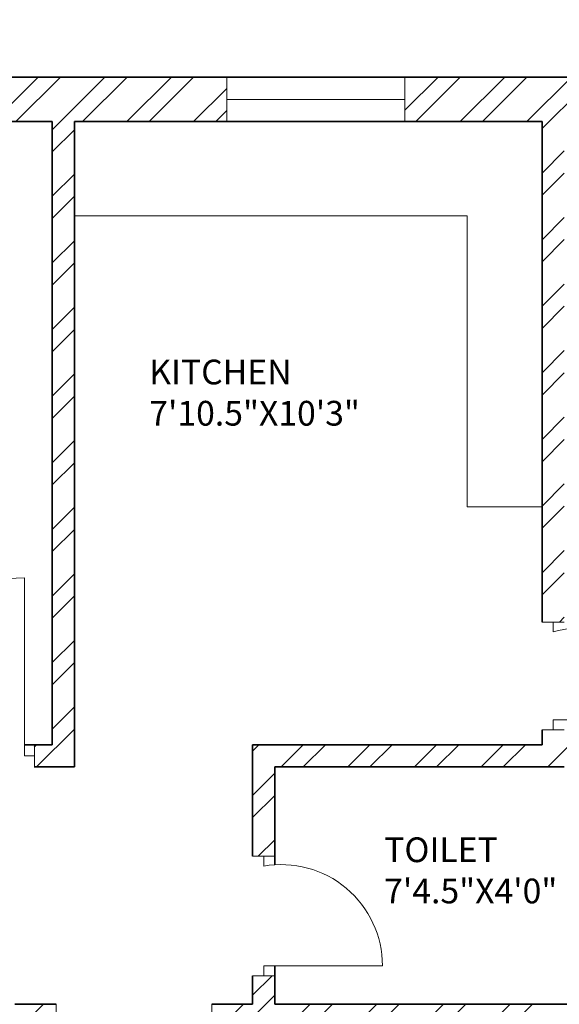
# Model space of a CAD drawing. Units: inches. Extents: x 2120 to 4013, y 1390 to 3019.
# Tile 44 of 59: x 2861 to 2970, y 2165 to 2364. Entities that reach past the tile are written whole.
import ezdxf

# ---------------------------------------------------------------- set-up
doc = ezdxf.new("R2010")
doc.units = ezdxf.units.IN
for name, color, linetype, lineweight in [('A-ANNO-DIMS', 2, 'Continuous', 18), ('A-AREA-IDEN', 7, 'Continuous', 18), ('A-DOOR', 3, 'Continuous', 18), ('A-FLOR-CASE', 8, 'Continuous', 18), ('A-GLAZ', 4, 'Continuous', 18), ('A-WALL', 7, 'Continuous', 35), ('A-WALL-PATT', 252, 'Continuous', 13)]:
    doc.layers.add(name, color=color, linetype=linetype, lineweight=lineweight)
doc.styles.get("Standard").update_dxf_attribs({"font": 'arial.ttf'})
doc.dimstyles.get("Standard").update_dxf_attribs({"dimtxt": 0.18, "dimasz": 0.18, "dimexe": 0.18, "dimexo": 0.0625, "dimgap": 0.09, "dimtad": 0, "dimtih": 1, "dimtoh": 1, "dimdec": 4, "dimzin": 0, "dimdsep": 46, "dimtxsty": 'Standard', "dimcen": 0.09, "dimadec": 0, "dimazin": 0, "dimtfac": 1, "dimtdec": 4, "dimtofl": 0, "dimtmove": 0, "dimatfit": 3, "dimfxl": 1, "dimtolj": 1, "dimtzin": 0, "dimarcsym": 0})

# ---------------------------------------------------------------- blocks, each defined once
blk = doc.blocks.new('DOOR-SWING-24IN-106p92DEG')
for p, q in [((4.5, 21.79), (0, 21.79)), ((0, 21.79), (2.25, 21.79)), ((2.25, 21.79), (2.25, 19.79)), ((2.25, 0), (2.25, 2)), ((2.25, 2), (26.25, 2)), ((0, 0), (4.5, 0)), ((4.5, 0), (2.25, 0))]:
    blk.add_line(p, q)
blk.add_arc((7.66, 2), 18.59, 0, 106.9181)
blk = doc.blocks.new('DOOR-SWING-24IN-99p98DEG')
for p, q in [((0, 24.15), (4.5, 24.15)), ((4.5, 24.15), (2.25, 24.15)), ((2.25, 24.15), (2.25, 22.15)), ((2.25, 0), (2.25, 2)), ((2.25, 2), (26.25, 2)), ((4.5, 0), (0, 0)), ((0, 0), (2.25, 0))]:
    blk.add_line(p, q)
blk.add_arc((5.79, 2), 20.46, 0, 99.9792)
blk = doc.blocks.new('DOOR-SWING-36IN-103p63DEG')
for p, q in [((30.32, 2.25), (30.32, 38.25)), ((0, 4.5), (0, 0)), ((32.32, 4.5), (32.32, 0)), ((0, 0), (0, 2.25)), ((0, 2.25), (2, 2.25)), ((32.32, 2.25), (30.32, 2.25)), ((32.32, 0), (32.32, 2.25))]:
    blk.add_line(p, q)
blk.add_arc((30.32, 9.11), 29.14, 90, 193.6269)
blk = doc.blocks.new('DOOR-SWING-36IN-105p32DEG')
for p, q in [((0, 33.75), (0, 38.25)), ((0, 38.25), (0, 36)), ((31.46, 33.75), (31.46, 38.25)), ((31.46, 38.25), (31.46, 36)), ((0, 36), (2, 36)), ((2, 36), (2, 0)), ((31.46, 36), (29.46, 36))]:
    blk.add_line(p, q)
blk.add_arc((2, 28.48), 28.48, 270, 15.3194)
blk = doc.blocks.new('WIN-PLAN-36IN')
for p, q in [((0, 0), (0, 9)), ((0, 9), (0, 4.5)), ((36, 4.5), (36, 9)), ((36, 9), (36, 0)), ((0, 4.5), (36, 4.5))]:
    blk.add_line(p, q)
blk = doc.blocks.new('*D211')
at = {"layer": 'A-ANNO-DIMS', "color": 0, "lineweight": -2, "transparency": 16777216}
for p, q in [((2262.73, 2352.59), (2262.73, 2397.71)), ((2262.91, 2397.53), (2635.95, 2397.53)), ((3009.55, 2397.53), (2636.52, 2397.53)), ((3009.73, 2352.59), (3009.73, 2397.71))]:
    blk.add_line(p, q, dxfattribs=at)
at = {"layer": 'A-ANNO-DIMS', "color": 0, "transparency": 16777216}
for points in [[(2262.91, 2397.56), (2262.91, 2397.5), (2262.73, 2397.53)], [(3009.55, 2397.56), (3009.55, 2397.5), (3009.73, 2397.53)]]:
    blk.add_solid(points, dxfattribs=at)
at = {"layer": 'Defpoints', "color": 0, "transparency": 16777216}
for p in [(3009.73, 2397.53), (2262.73, 2352.53), (3009.73, 2352.53)]:
    blk.add_point(p, dxfattribs=at)
at = {"layer": 'A-ANNO-DIMS', "color": 0, "transparency": 16777216, "insert": (2636.23, 2397.53), "char_height": 0.18, "attachment_point": 5}
blk.add_mtext('\\A1;747', dxfattribs=at)

msp = doc.modelspace()

# ---------------------------------------------------------------- hatches: boundary and pattern name
at = {"layer": 'A-WALL-PATT'}
h = msp.add_hatch(dxfattribs=at)
h.set_pattern_fill('ANSI32', color=256)
h.paths.add_polyline_path([(2271.7331, 2343.531), (2283.3788, 2343.531), (2283.3788, 2348.031), (2283.3788, 2352.5306), (2262.7331, 2352.5306), (2262.7331, 2182.638), (2267.2331, 2182.638), (2271.7331, 2182.638), (2271.7331, 2219.031), (2391.7331, 2219.031), (2391.7331, 2214.189), (2393.9831, 2214.189), (2396.2331, 2214.189), (2396.2331, 2219.031), (2420.2331, 2219.031), (2420.2331, 2225.7535), (2417.2197, 2225.7535), (2415.7331, 2225.7535), (2415.7331, 2223.5306), (2271.7331, 2223.5306)])
h.paths.add_polyline_path([(2380.0942, 2352.5306), (2343.3788, 2352.5306), (2343.3788, 2343.531), (2363.2331, 2343.531), (2363.2331, 2288.8489), (2365.4831, 2288.8489), (2367.7331, 2288.8489), (2367.7331, 2343.531), (2380.0942, 2343.531)], flags=17)
h.paths.add_polyline_path([(2432.4339, 2352.5306), (2404.0943, 2352.5306), (2404.0943, 2343.531), (2415.7331, 2343.531), (2415.7331, 2264.0306), (2367.7331, 2264.0306), (2367.7331, 2266.4872), (2363.2331, 2266.4872), (2363.2331, 2259.531), (2367.7331, 2259.531), (2415.7331, 2259.531), (2415.7331, 2255.0658), (2420.2331, 2255.0658), (2420.2331, 2259.531), (2424.5717, 2259.531), (2424.5717, 2261.781), (2424.5717, 2264.0306), (2420.2331, 2264.0306), (2420.2331, 2343.531), (2432.4339, 2343.531)])
h.paths.add_polyline_path([(2508.9115, 2352.5306), (2456.4339, 2352.5306), (2456.4339, 2343.531), (2468.2331, 2343.531), (2468.2331, 2264.0306), (2448.0487, 2264.0306), (2448.0487, 2259.531), (2468.2331, 2259.531), (2468.2331, 2255.5496), (2472.7331, 2255.5496), (2472.7331, 2343.531), (2508.9115, 2343.531)])
h.paths.add_polyline_path([(2637.7331, 2352.5306), (2544.9116, 2352.5306), (2544.9116, 2343.531), (2589.7331, 2343.531), (2633.2331, 2343.531), (2637.7331, 2343.531)])
h.paths.add_polyline_path([(2594.2331, 2343.5306), (2589.7331, 2343.5306), (2589.7331, 2259.5306), (2589.7331, 2252.4915), (2591.9831, 2252.4915), (2594.2331, 2252.4915)])
h.paths.add_polyline_path([(2637.7331, 2223.5306), (2594.2331, 2223.5306), (2594.2331, 2230.1988), (2591.9831, 2230.1988), (2589.7331, 2230.1988), (2589.7331, 2223.5306), (2472.7331, 2223.5306), (2468.2331, 2223.5306), (2468.2331, 2219.031), (2628.7331, 2219.031), (2628.7331, 2138.031), (2637.7331, 2138.031)])
h.paths.add_polyline_path([(3822.6535, 2458.4402), (3874.9468, 2458.4402), (3874.9468, 2476.9866), (3822.6535, 2476.9866)], flags=9)
h.paths.add_polyline_path([(3834.6921, 2781.8174), (3935.9206, 2781.8174), (3935.9206, 2800.3638), (3834.6921, 2800.3638)], flags=9)
h.paths.add_polyline_path([(3832.2843, 2837.9683), (3884.5776, 2837.9683), (3884.5776, 2856.5146), (3832.2843, 2856.5146)], flags=9)
h.paths.add_polyline_path([(3830.9388, 2861.4782), (3956.8958, 2861.4782), (3956.8958, 2880.0245), (3830.9388, 2880.0245)], flags=9)
h.paths.add_polyline_path([(3870.6966, 2352.5752), (3887.9272, 2352.5752), (3887.9272, 2377.3037), (3870.6966, 2377.3037)], flags=9)
h.paths.add_polyline_path([(3289.2701, 2413.161), (3435.2223, 2413.161), (3435.2223, 2450.2538), (3289.2701, 2450.2538)], flags=9)
h.paths.add_polyline_path([(2487.6944, 2414.3601), (2637.8335, 2414.3601), (2637.8335, 2451.4528), (2487.6944, 2451.4528)], flags=9)
h.paths.add_polyline_path([(2567.3724, 1457.9199), (2815.296, 1457.9199), (2815.296, 1495.0127), (2567.3724, 1495.0127)], flags=9)
h.paths.add_polyline_path([(2655.3825, 2093.2363), (2685.9555, 2093.2363), (2685.9555, 2111.8937), (2655.3825, 2111.8937)], flags=9)
h.paths.add_polyline_path([(2543.9218, 1550.6671), (2587.8406, 1550.6671), (2587.8406, 1569.3244), (2543.9218, 1569.3244)], flags=9)
h.paths.add_polyline_path([(2905.1384, 1543.8113), (2949.0572, 1543.8113), (2949.0572, 1562.4686), (2905.1384, 1562.4686)], flags=9)
h.paths.add_polyline_path([(2736.4118, 1702.4736), (2784.2153, 1702.4736), (2784.2153, 1721.1309), (2736.4118, 1721.1309)], flags=9)
h.paths.add_polyline_path([(2912.8666, 1710.4168), (2951.707, 1710.4168), (2951.707, 1729.0741), (2912.8666, 1729.0741)], flags=9)
h.paths.add_polyline_path([(2923.5785, 1763.5038), (2959.7279, 1763.5038), (2959.7279, 1782.1611), (2923.5785, 1782.1611)], flags=9)
h.paths.add_polyline_path([(2925.2114, 1809.6137), (2967.1861, 1809.6137), (2967.1861, 1828.271), (2925.2114, 1828.271)], flags=9)
h.paths.add_polyline_path([(2996.2711, 1878.9003), (2996.2711, 1913.109), (2977.6138, 1913.109), (2977.6138, 1878.9003)], flags=9)
h.paths.add_polyline_path([(2883.0859, 1895.7192), (2927.1855, 1895.7192), (2927.1855, 1914.3766), (2883.0859, 1914.3766)], flags=9)
h.paths.add_polyline_path([(2787.3924, 1810.8013), (2841.0213, 1810.8013), (2841.0213, 1829.4587), (2787.3924, 1829.4587)], flags=9)
h.paths.add_polyline_path([(2775.6399, 2101.7395), (2829.2689, 2101.7395), (2829.2689, 2120.3968), (2775.6399, 2120.3968)], flags=9)
h.paths.add_polyline_path([(2913.0263, 2075.817), (2951.8667, 2075.817), (2951.8667, 2094.4744), (2913.0263, 2094.4744)], flags=9)
h.paths.add_polyline_path([(2929.966, 2133.3669), (2966.1154, 2133.3669), (2966.1154, 2152.0243), (2929.966, 2152.0243)], flags=9)
h.paths.add_polyline_path([(2932.7502, 2182.6088), (2968.8996, 2182.6088), (2968.8996, 2201.2662), (2932.7502, 2201.2662)], flags=9)
h.paths.add_polyline_path([(2996.0681, 2266.3173), (2996.0681, 2300.5261), (2977.4108, 2300.5261), (2977.4108, 2266.3173)], flags=9)
h.paths.add_polyline_path([(2885.1039, 2279.2186), (2929.2035, 2279.2186), (2929.2035, 2297.8759), (2885.1039, 2297.8759)], flags=9)
h.paths.add_polyline_path([(2735.7042, 2218.3197), (2783.5078, 2218.3197), (2783.5078, 2236.9771), (2735.7042, 2236.9771)], flags=9)
h.paths.add_polyline_path([(2635.6049, 2044.0085), (2648.9678, 2044.0085), (2648.9678, 2054.312), (2635.6049, 2054.312)], flags=9)
h.paths.add_polyline_path([(2714.0148, 1923.0473), (2727.3777, 1923.0473), (2727.3777, 1933.3508), (2714.0148, 1933.3508)], flags=9)
h.paths.add_polyline_path([(2709.0345, 1988.1628), (2722.3974, 1988.1628), (2722.3974, 1998.4663), (2709.0345, 1998.4663)], flags=9)
h.paths.add_polyline_path([(2592.8935, 1962.1763), (2606.2564, 1962.1763), (2606.2564, 1972.4799), (2592.8935, 1972.4799)], flags=9)
h.paths.add_polyline_path([(2618.3996, 1985.9724), (2644.1942, 1985.9724), (2644.1942, 1996.2759), (2618.3996, 1996.2759)], flags=9)
h.paths.add_polyline_path([(2601.279, 1920.5869), (2614.6419, 1920.5869), (2614.6419, 1930.8904), (2601.279, 1930.8904)], flags=9)
h.paths.add_polyline_path([(2692.3278, 1932.7645), (2704.5311, 1932.7645), (2704.5311, 1943.0681), (2692.3278, 1943.0681)], flags=9)
h.paths.add_polyline_path([(2311.122, 1672.7318), (2355.0408, 1672.7318), (2355.0408, 1691.3892), (2311.122, 1691.3892)], flags=9)
h.paths.add_polyline_path([(2456.2551, 1632.3198), (2492.4796, 1632.3198), (2492.4796, 1650.9772), (2456.2551, 1650.9772)], flags=9)
h.paths.add_polyline_path([(2401.0766, 1631.4793), (2437.301, 1631.4793), (2437.301, 1650.1367), (2401.0766, 1650.1367)], flags=9)
h.paths.add_polyline_path([(2546.7054, 1700.9235), (2594.509, 1700.9235), (2594.509, 1719.5809), (2546.7054, 1719.5809)], flags=9)
h.paths.add_polyline_path([(2445.4866, 1766.9937), (2497.5261, 1766.9937), (2497.5261, 1785.651), (2445.4866, 1785.651)], flags=9)
h.paths.add_polyline_path([(2287.9992, 1739.7675), (2326.8396, 1739.7675), (2326.8396, 1758.4248), (2287.9992, 1758.4248)], flags=9)
h.paths.add_polyline_path([(2458.5279, 1924.7607), (2510.5675, 1924.7607), (2510.5675, 1943.4181), (2458.5279, 1943.4181)], flags=9)
h.paths.add_polyline_path([(2309.2811, 1902.7642), (2345.4305, 1902.7642), (2345.4305, 1921.4215), (2309.2811, 1921.4215)], flags=9)
h.paths.add_polyline_path([(2490.7554, 2018.9392), (2530.7896, 2018.9392), (2530.7896, 2037.5965), (2490.7554, 2037.5965)], flags=9)
h.paths.add_polyline_path([(2402.143, 2024.7393), (2438.5414, 2024.7393), (2438.5414, 2043.3966), (2402.143, 2043.3966)], flags=9)
h.paths.add_polyline_path([(2287.856, 1931.7926), (2326.6964, 1931.7926), (2326.6964, 1950.4499), (2287.856, 1950.4499)], flags=9)
h.paths.add_polyline_path([(2281.7979, 2193.5771), (2320.6383, 2193.5771), (2320.6383, 2212.2344), (2281.7979, 2212.2344)], flags=25)
h.paths.add_polyline_path([(2484.0754, 2093.892), (2536.115, 2093.892), (2536.115, 2112.5494), (2484.0754, 2112.5494)], flags=9)
h.paths.add_polyline_path([(2624.7948, 2281.8639), (2624.7948, 2311.4137), (2606.1375, 2311.4137), (2606.1375, 2281.8639)], flags=9)
h.paths.add_polyline_path([(2507.5036, 2290.3639), (2541.934, 2290.3639), (2541.934, 2309.0212), (2507.5036, 2309.0212)], flags=9)
h.paths.add_polyline_path([(2423.1076, 2285.2202), (2459.332, 2285.2202), (2459.332, 2303.8776), (2423.1076, 2303.8776)], flags=9)
h.paths.add_polyline_path([(2374.5467, 2289.6272), (2410.7711, 2289.6272), (2410.7711, 2308.2846), (2374.5467, 2308.2846)], flags=25)
h.paths.add_polyline_path([(2277.4907, 2227.5651), (2316.3311, 2227.5651), (2316.3311, 2246.2224), (2277.4907, 2246.2224)], flags=25)
h.paths.add_polyline_path([(2655.3825, 2093.2367), (2685.9555, 2093.2367), (2685.9555, 2111.894), (2655.3825, 2111.894)], flags=9)
h.paths.add_polyline_path([(2543.9217, 1550.6674), (2587.8406, 1550.6674), (2587.8406, 1569.3247), (2543.9217, 1569.3247)], flags=9)
h.paths.add_polyline_path([(2905.1384, 1543.8116), (2949.0572, 1543.8116), (2949.0572, 1562.4689), (2905.1384, 1562.4689)], flags=9)
h.paths.add_polyline_path([(2736.4118, 1702.4739), (2784.2153, 1702.4739), (2784.2153, 1721.1312), (2736.4118, 1721.1312)], flags=9)
h.paths.add_polyline_path([(2912.8666, 1710.4171), (2951.707, 1710.4171), (2951.707, 1729.0744), (2912.8666, 1729.0744)], flags=9)
h.paths.add_polyline_path([(2923.5785, 1763.5041), (2959.7279, 1763.5041), (2959.7279, 1782.1614), (2923.5785, 1782.1614)], flags=9)
h.paths.add_polyline_path([(2925.2114, 1809.614), (2967.1861, 1809.614), (2967.1861, 1828.2713), (2925.2114, 1828.2713)], flags=9)
h.paths.add_polyline_path([(2996.2711, 1878.9006), (2996.2711, 1913.1094), (2977.6137, 1913.1094), (2977.6137, 1878.9006)], flags=9)
h.paths.add_polyline_path([(2883.0859, 1895.7195), (2927.1855, 1895.7195), (2927.1855, 1914.3769), (2883.0859, 1914.3769)], flags=9)
h.paths.add_polyline_path([(2787.3924, 1810.8016), (2841.0213, 1810.8016), (2841.0213, 1829.459), (2787.3924, 1829.459)], flags=9)
h.paths.add_polyline_path([(2775.6399, 2101.7398), (2829.2688, 2101.7398), (2829.2688, 2120.3971), (2775.6399, 2120.3971)], flags=9)
h.paths.add_polyline_path([(2913.0263, 2075.8173), (2951.8667, 2075.8173), (2951.8667, 2094.4747), (2913.0263, 2094.4747)], flags=9)
h.paths.add_polyline_path([(2929.966, 2133.3672), (2966.1154, 2133.3672), (2966.1154, 2152.0246), (2929.966, 2152.0246)], flags=9)
h.paths.add_polyline_path([(2932.7502, 2182.6091), (2968.8996, 2182.6091), (2968.8996, 2201.2665), (2932.7502, 2201.2665)], flags=9)
h.paths.add_polyline_path([(2996.0681, 2266.3176), (2996.0681, 2300.5264), (2977.4108, 2300.5264), (2977.4108, 2266.3176)], flags=9)
h.paths.add_polyline_path([(2885.1039, 2279.2189), (2929.2035, 2279.2189), (2929.2035, 2297.8762), (2885.1039, 2297.8762)], flags=9)
h.paths.add_polyline_path([(2735.7042, 2218.32), (2783.5078, 2218.32), (2783.5078, 2236.9774), (2735.7042, 2236.9774)], flags=9)
h.paths.add_polyline_path([(2635.6048, 2044.0088), (2648.9677, 2044.0088), (2648.9677, 2054.3123), (2635.6048, 2054.3123)], flags=9)
h.paths.add_polyline_path([(2714.0148, 1923.0476), (2727.3777, 1923.0476), (2727.3777, 1933.3511), (2714.0148, 1933.3511)], flags=9)
h.paths.add_polyline_path([(2709.0345, 1988.1631), (2722.3974, 1988.1631), (2722.3974, 1998.4666), (2709.0345, 1998.4666)], flags=9)
h.paths.add_polyline_path([(2592.8935, 1962.1766), (2606.2564, 1962.1766), (2606.2564, 1972.4802), (2592.8935, 1972.4802)], flags=9)
h.paths.add_polyline_path([(2618.3995, 1985.9727), (2644.1942, 1985.9727), (2644.1942, 1996.2762), (2618.3995, 1996.2762)], flags=9)
h.paths.add_polyline_path([(2601.279, 1920.5872), (2614.6419, 1920.5872), (2614.6419, 1930.8908), (2601.279, 1930.8908)], flags=9)
h.paths.add_polyline_path([(2692.3278, 1932.7648), (2704.5311, 1932.7648), (2704.5311, 1943.0684), (2692.3278, 1943.0684)], flags=9)
h.paths.add_polyline_path([(2311.122, 1672.7321), (2355.0408, 1672.7321), (2355.0408, 1691.3895), (2311.122, 1691.3895)], flags=9)
h.paths.add_polyline_path([(2456.2551, 1632.3201), (2492.4795, 1632.3201), (2492.4795, 1650.9775), (2456.2551, 1650.9775)], flags=9)
h.paths.add_polyline_path([(2401.0766, 1631.4796), (2437.301, 1631.4796), (2437.301, 1650.137), (2401.0766, 1650.137)], flags=9)
h.paths.add_polyline_path([(2546.7054, 1700.9238), (2594.509, 1700.9238), (2594.509, 1719.5812), (2546.7054, 1719.5812)], flags=9)
h.paths.add_polyline_path([(2445.4866, 1766.994), (2497.5261, 1766.994), (2497.5261, 1785.6513), (2445.4866, 1785.6513)], flags=9)
h.paths.add_polyline_path([(2287.9992, 1739.7678), (2326.8396, 1739.7678), (2326.8396, 1758.4251), (2287.9992, 1758.4251)], flags=9)
h.paths.add_polyline_path([(2458.5279, 1924.7611), (2510.5675, 1924.7611), (2510.5675, 1943.4184), (2458.5279, 1943.4184)], flags=9)
h.paths.add_polyline_path([(2309.2811, 1902.7645), (2345.4305, 1902.7645), (2345.4305, 1921.4218), (2309.2811, 1921.4218)], flags=9)
h.paths.add_polyline_path([(2490.7554, 2018.9395), (2530.7895, 2018.9395), (2530.7895, 2037.5968), (2490.7554, 2037.5968)], flags=9)
h.paths.add_polyline_path([(2402.143, 2024.7396), (2438.5413, 2024.7396), (2438.5413, 2043.3969), (2402.143, 2043.3969)], flags=9)
h.paths.add_polyline_path([(2287.856, 1931.7929), (2326.6964, 1931.7929), (2326.6964, 1950.4502), (2287.856, 1950.4502)], flags=9)
h.paths.add_polyline_path([(2281.7979, 2193.5774), (2320.6383, 2193.5774), (2320.6383, 2212.2347), (2281.7979, 2212.2347)], flags=25)
h.paths.add_polyline_path([(2484.0754, 2093.8924), (2536.115, 2093.8924), (2536.115, 2112.5497), (2484.0754, 2112.5497)], flags=9)
h.paths.add_polyline_path([(2624.7948, 2281.8642), (2624.7948, 2311.414), (2606.1374, 2311.414), (2606.1374, 2281.8642)], flags=9)
h.paths.add_polyline_path([(2507.5035, 2290.3642), (2541.934, 2290.3642), (2541.934, 2309.0215), (2507.5035, 2309.0215)], flags=9)
h.paths.add_polyline_path([(2423.1075, 2285.2205), (2459.332, 2285.2205), (2459.332, 2303.8779), (2423.1075, 2303.8779)], flags=9)
h.paths.add_polyline_path([(2374.5467, 2289.6275), (2410.7711, 2289.6275), (2410.7711, 2308.2849), (2374.5467, 2308.2849)], flags=25)
h.paths.add_polyline_path([(2277.4907, 2227.5654), (2316.3311, 2227.5654), (2316.3311, 2246.2227), (2277.4907, 2246.2227)], flags=25)
h = msp.add_hatch(dxfattribs=at)
h.set_pattern_fill('ANSI32', color=256)
h.paths.add_polyline_path([(2271.7331, 1980.389), (2262.7331, 1980.389), (2262.7331, 1912.8434), (2267.2331, 1912.8434), (2271.7331, 1912.8434), (2271.7331, 1922.531), (2351.2331, 1922.531), (2351.2331, 1901.4728), (2355.7331, 1901.4728), (2355.7331, 1922.531), (2357.9815, 1922.531), (2357.9815, 1926.5306), (2271.7331, 1926.5306)])
h.paths.add_polyline_path([(2589.2331, 1949.1622), (2584.7331, 1949.1622), (2580.2331, 1949.1622), (2580.2331, 1874.5306), (2355.7331, 1874.5306), (2355.7331, 1880.1922), (2351.2331, 1880.1922), (2351.2331, 1874.5306), (2271.7331, 1874.5306), (2271.7331, 1888.8431), (2262.7331, 1888.8431), (2262.7331, 1842.2909), (2267.2331, 1842.2909), (2271.7331, 1842.2909), (2271.7331, 1865.531), (2415.7331, 1865.531), (2415.7331, 1779.7286), (2420.2331, 1779.7286), (2420.2331, 1865.531), (2589.2331, 1865.531)])
h.paths.add_polyline_path([(2271.7331, 1782.2906), (2262.7331, 1782.2906), (2262.7331, 1711.4639), (2267.2331, 1711.4639), (2271.7331, 1711.4639), (2271.7331, 1738.031), (2420.2331, 1738.031), (2420.2331, 1742.531), (2420.2331, 1747.3376), (2417.9831, 1747.3376), (2415.7331, 1747.3376), (2415.7331, 1742.5306), (2271.7331, 1742.5306)])
h.paths.add_polyline_path([(2271.7331, 1627.031), (2362.3957, 1627.031), (2362.3957, 1629.281), (2362.3957, 1631.5306), (2271.7331, 1631.5306), (2271.7331, 1675.4636), (2262.7331, 1675.4636), (2262.7331, 1581.531), (2405.3032, 1581.531), (2405.3032, 1586.031), (2405.3032, 1590.5306), (2396.2331, 1590.5306), (2396.2331, 1691.4513), (2418.7206, 1691.4513), (2418.7206, 1695.951), (2396.2331, 1695.951), (2391.7331, 1695.951), (2391.7331, 1631.5306), (2386.7425, 1631.5306), (2386.7425, 1629.2806), (2386.7425, 1627.031), (2391.7331, 1627.031), (2391.7331, 1586.1709), (2271.7331, 1586.1709)])
h.paths.add_polyline_path([(2459.6703, 1590.5306), (2429.3032, 1590.5306), (2429.3032, 1581.531), (2459.6703, 1581.531), (2459.6703, 1586.031)])
h.paths.add_polyline_path([(2501.2331, 1590.531), (2501.2331, 1665.0195), (2498.9831, 1665.0195), (2496.7331, 1665.0195), (2496.7331, 1590.5306), (2483.8201, 1590.5306), (2483.8201, 1590.1579), (2483.6704, 1590.1579), (2483.6704, 1581.531), (2505.0196, 1581.531), (2505.0196, 1583.781), (2505.0196, 1586.0306), (2501.2331, 1586.0306)])
h.paths.add_polyline_path([(2544.1361, 1583.781), (2544.1361, 1586.0306), (2527.1368, 1586.0306), (2527.1368, 1583.7806), (2527.1368, 1581.531), (2544.1361, 1581.531)])
h.paths.add_polyline_path([(3822.6535, 2458.4402), (3874.9468, 2458.4402), (3874.9468, 2476.9866), (3822.6535, 2476.9866)], flags=9)
h.paths.add_polyline_path([(3834.6921, 2781.8174), (3935.9206, 2781.8174), (3935.9206, 2800.3638), (3834.6921, 2800.3638)], flags=9)
h.paths.add_polyline_path([(3832.2843, 2837.9683), (3884.5776, 2837.9683), (3884.5776, 2856.5146), (3832.2843, 2856.5146)], flags=9)
h.paths.add_polyline_path([(3830.9388, 2861.4782), (3956.8958, 2861.4782), (3956.8958, 2880.0245), (3830.9388, 2880.0245)], flags=9)
h.paths.add_polyline_path([(3870.6966, 2352.5752), (3887.9272, 2352.5752), (3887.9272, 2377.3037), (3870.6966, 2377.3037)], flags=9)
h.paths.add_polyline_path([(3289.2701, 2413.161), (3435.2223, 2413.161), (3435.2223, 2450.2538), (3289.2701, 2450.2538)], flags=9)
h.paths.add_polyline_path([(2487.6944, 2414.3601), (2637.8335, 2414.3601), (2637.8335, 2451.4528), (2487.6944, 2451.4528)], flags=9)
h.paths.add_polyline_path([(2567.3724, 1457.9199), (2815.296, 1457.9199), (2815.296, 1495.0127), (2567.3724, 1495.0127)], flags=9)
h.paths.add_polyline_path([(2655.3825, 2093.2363), (2685.9555, 2093.2363), (2685.9555, 2111.8937), (2655.3825, 2111.8937)], flags=9)
h.paths.add_polyline_path([(2543.9218, 1550.6671), (2587.8406, 1550.6671), (2587.8406, 1569.3244), (2543.9218, 1569.3244)], flags=9)
h.paths.add_polyline_path([(2905.1384, 1543.8113), (2949.0572, 1543.8113), (2949.0572, 1562.4686), (2905.1384, 1562.4686)], flags=9)
h.paths.add_polyline_path([(2736.4118, 1702.4736), (2784.2153, 1702.4736), (2784.2153, 1721.1309), (2736.4118, 1721.1309)], flags=9)
h.paths.add_polyline_path([(2912.8666, 1710.4168), (2951.707, 1710.4168), (2951.707, 1729.0741), (2912.8666, 1729.0741)], flags=9)
h.paths.add_polyline_path([(2923.5785, 1763.5038), (2959.7279, 1763.5038), (2959.7279, 1782.1611), (2923.5785, 1782.1611)], flags=9)
h.paths.add_polyline_path([(2925.2114, 1809.6137), (2967.1861, 1809.6137), (2967.1861, 1828.271), (2925.2114, 1828.271)], flags=9)
h.paths.add_polyline_path([(2996.2711, 1878.9003), (2996.2711, 1913.109), (2977.6138, 1913.109), (2977.6138, 1878.9003)], flags=9)
h.paths.add_polyline_path([(2883.0859, 1895.7192), (2927.1855, 1895.7192), (2927.1855, 1914.3766), (2883.0859, 1914.3766)], flags=9)
h.paths.add_polyline_path([(2787.3924, 1810.8013), (2841.0213, 1810.8013), (2841.0213, 1829.4587), (2787.3924, 1829.4587)], flags=9)
h.paths.add_polyline_path([(2775.6399, 2101.7395), (2829.2689, 2101.7395), (2829.2689, 2120.3968), (2775.6399, 2120.3968)], flags=9)
h.paths.add_polyline_path([(2913.0263, 2075.817), (2951.8667, 2075.817), (2951.8667, 2094.4744), (2913.0263, 2094.4744)], flags=9)
h.paths.add_polyline_path([(2929.966, 2133.3669), (2966.1154, 2133.3669), (2966.1154, 2152.0243), (2929.966, 2152.0243)], flags=9)
h.paths.add_polyline_path([(2932.7502, 2182.6088), (2968.8996, 2182.6088), (2968.8996, 2201.2662), (2932.7502, 2201.2662)], flags=9)
h.paths.add_polyline_path([(2996.0681, 2266.3173), (2996.0681, 2300.5261), (2977.4108, 2300.5261), (2977.4108, 2266.3173)], flags=9)
h.paths.add_polyline_path([(2885.1039, 2279.2186), (2929.2035, 2279.2186), (2929.2035, 2297.8759), (2885.1039, 2297.8759)], flags=9)
h.paths.add_polyline_path([(2735.7042, 2218.3197), (2783.5078, 2218.3197), (2783.5078, 2236.9771), (2735.7042, 2236.9771)], flags=9)
h.paths.add_polyline_path([(2635.6049, 2044.0085), (2648.9678, 2044.0085), (2648.9678, 2054.312), (2635.6049, 2054.312)], flags=9)
h.paths.add_polyline_path([(2714.0148, 1923.0473), (2727.3777, 1923.0473), (2727.3777, 1933.3508), (2714.0148, 1933.3508)], flags=9)
h.paths.add_polyline_path([(2709.0345, 1988.1628), (2722.3974, 1988.1628), (2722.3974, 1998.4663), (2709.0345, 1998.4663)], flags=9)
h.paths.add_polyline_path([(2592.8935, 1962.1763), (2606.2564, 1962.1763), (2606.2564, 1972.4799), (2592.8935, 1972.4799)], flags=9)
h.paths.add_polyline_path([(2618.3996, 1985.9724), (2644.1942, 1985.9724), (2644.1942, 1996.2759), (2618.3996, 1996.2759)], flags=9)
h.paths.add_polyline_path([(2601.279, 1920.5869), (2614.6419, 1920.5869), (2614.6419, 1930.8904), (2601.279, 1930.8904)], flags=9)
h.paths.add_polyline_path([(2692.3278, 1932.7645), (2704.5311, 1932.7645), (2704.5311, 1943.0681), (2692.3278, 1943.0681)], flags=9)
h.paths.add_polyline_path([(2311.122, 1672.7318), (2355.0408, 1672.7318), (2355.0408, 1691.3892), (2311.122, 1691.3892)], flags=25)
h.paths.add_polyline_path([(2456.2551, 1632.3198), (2492.4796, 1632.3198), (2492.4796, 1650.9772), (2456.2551, 1650.9772)], flags=9)
h.paths.add_polyline_path([(2401.0766, 1631.4793), (2437.301, 1631.4793), (2437.301, 1650.1367), (2401.0766, 1650.1367)], flags=9)
h.paths.add_polyline_path([(2546.7054, 1700.9235), (2594.509, 1700.9235), (2594.509, 1719.5809), (2546.7054, 1719.5809)], flags=9)
h.paths.add_polyline_path([(2445.4866, 1766.9937), (2497.5261, 1766.9937), (2497.5261, 1785.651), (2445.4866, 1785.651)], flags=9)
h.paths.add_polyline_path([(2287.9992, 1739.7675), (2326.8396, 1739.7675), (2326.8396, 1758.4248), (2287.9992, 1758.4248)], flags=24)
h.paths.add_polyline_path([(2458.5279, 1924.7607), (2510.5675, 1924.7607), (2510.5675, 1943.4181), (2458.5279, 1943.4181)], flags=25)
h.paths.add_polyline_path([(2309.2811, 1902.7642), (2345.4305, 1902.7642), (2345.4305, 1921.4215), (2309.2811, 1921.4215)], flags=25)
h.paths.add_polyline_path([(2490.7554, 2018.9392), (2530.7896, 2018.9392), (2530.7896, 2037.5965), (2490.7554, 2037.5965)], flags=9)
h.paths.add_polyline_path([(2402.143, 2024.7393), (2438.5414, 2024.7393), (2438.5414, 2043.3966), (2402.143, 2043.3966)], flags=9)
h.paths.add_polyline_path([(2287.856, 1931.7926), (2326.6964, 1931.7926), (2326.6964, 1950.4499), (2287.856, 1950.4499)], flags=25)
h.paths.add_polyline_path([(2281.7979, 2193.5771), (2320.6383, 2193.5771), (2320.6383, 2212.2344), (2281.7979, 2212.2344)], flags=9)
h.paths.add_polyline_path([(2484.0754, 2093.892), (2536.115, 2093.892), (2536.115, 2112.5494), (2484.0754, 2112.5494)], flags=9)
h.paths.add_polyline_path([(2624.7948, 2281.8639), (2624.7948, 2311.4137), (2606.1375, 2311.4137), (2606.1375, 2281.8639)], flags=9)
h.paths.add_polyline_path([(2507.5036, 2290.3639), (2541.934, 2290.3639), (2541.934, 2309.0212), (2507.5036, 2309.0212)], flags=9)
h.paths.add_polyline_path([(2423.1076, 2285.2202), (2459.332, 2285.2202), (2459.332, 2303.8776), (2423.1076, 2303.8776)], flags=9)
h.paths.add_polyline_path([(2374.5467, 2289.6272), (2410.7711, 2289.6272), (2410.7711, 2308.2846), (2374.5467, 2308.2846)], flags=9)
h.paths.add_polyline_path([(2277.4907, 2227.5651), (2316.3311, 2227.5651), (2316.3311, 2246.2224), (2277.4907, 2246.2224)], flags=9)
h.paths.add_polyline_path([(2655.3825, 2093.2367), (2685.9555, 2093.2367), (2685.9555, 2111.894), (2655.3825, 2111.894)], flags=9)
h.paths.add_polyline_path([(2543.9217, 1550.6674), (2587.8406, 1550.6674), (2587.8406, 1569.3247), (2543.9217, 1569.3247)], flags=9)
h.paths.add_polyline_path([(2905.1384, 1543.8116), (2949.0572, 1543.8116), (2949.0572, 1562.4689), (2905.1384, 1562.4689)], flags=9)
h.paths.add_polyline_path([(2736.4118, 1702.4739), (2784.2153, 1702.4739), (2784.2153, 1721.1312), (2736.4118, 1721.1312)], flags=9)
h.paths.add_polyline_path([(2912.8666, 1710.4171), (2951.707, 1710.4171), (2951.707, 1729.0744), (2912.8666, 1729.0744)], flags=9)
h.paths.add_polyline_path([(2923.5785, 1763.5041), (2959.7279, 1763.5041), (2959.7279, 1782.1614), (2923.5785, 1782.1614)], flags=9)
h.paths.add_polyline_path([(2925.2114, 1809.614), (2967.1861, 1809.614), (2967.1861, 1828.2713), (2925.2114, 1828.2713)], flags=9)
h.paths.add_polyline_path([(2996.2711, 1878.9006), (2996.2711, 1913.1094), (2977.6137, 1913.1094), (2977.6137, 1878.9006)], flags=9)
h.paths.add_polyline_path([(2883.0859, 1895.7195), (2927.1855, 1895.7195), (2927.1855, 1914.3769), (2883.0859, 1914.3769)], flags=9)
h.paths.add_polyline_path([(2787.3924, 1810.8016), (2841.0213, 1810.8016), (2841.0213, 1829.459), (2787.3924, 1829.459)], flags=9)
h.paths.add_polyline_path([(2775.6399, 2101.7398), (2829.2688, 2101.7398), (2829.2688, 2120.3971), (2775.6399, 2120.3971)], flags=9)
h.paths.add_polyline_path([(2913.0263, 2075.8173), (2951.8667, 2075.8173), (2951.8667, 2094.4747), (2913.0263, 2094.4747)], flags=9)
h.paths.add_polyline_path([(2929.966, 2133.3672), (2966.1154, 2133.3672), (2966.1154, 2152.0246), (2929.966, 2152.0246)], flags=9)
h.paths.add_polyline_path([(2932.7502, 2182.6091), (2968.8996, 2182.6091), (2968.8996, 2201.2665), (2932.7502, 2201.2665)], flags=9)
h.paths.add_polyline_path([(2996.0681, 2266.3176), (2996.0681, 2300.5264), (2977.4108, 2300.5264), (2977.4108, 2266.3176)], flags=9)
h.paths.add_polyline_path([(2885.1039, 2279.2189), (2929.2035, 2279.2189), (2929.2035, 2297.8762), (2885.1039, 2297.8762)], flags=9)
h.paths.add_polyline_path([(2735.7042, 2218.32), (2783.5078, 2218.32), (2783.5078, 2236.9774), (2735.7042, 2236.9774)], flags=9)
h.paths.add_polyline_path([(2635.6048, 2044.0088), (2648.9677, 2044.0088), (2648.9677, 2054.3123), (2635.6048, 2054.3123)], flags=9)
h.paths.add_polyline_path([(2714.0148, 1923.0476), (2727.3777, 1923.0476), (2727.3777, 1933.3511), (2714.0148, 1933.3511)], flags=9)
h.paths.add_polyline_path([(2709.0345, 1988.1631), (2722.3974, 1988.1631), (2722.3974, 1998.4666), (2709.0345, 1998.4666)], flags=9)
h.paths.add_polyline_path([(2592.8935, 1962.1766), (2606.2564, 1962.1766), (2606.2564, 1972.4802), (2592.8935, 1972.4802)], flags=9)
h.paths.add_polyline_path([(2618.3995, 1985.9727), (2644.1942, 1985.9727), (2644.1942, 1996.2762), (2618.3995, 1996.2762)], flags=9)
h.paths.add_polyline_path([(2601.279, 1920.5872), (2614.6419, 1920.5872), (2614.6419, 1930.8908), (2601.279, 1930.8908)], flags=9)
h.paths.add_polyline_path([(2692.3278, 1932.7648), (2704.5311, 1932.7648), (2704.5311, 1943.0684), (2692.3278, 1943.0684)], flags=9)
h.paths.add_polyline_path([(2311.122, 1672.7321), (2355.0408, 1672.7321), (2355.0408, 1691.3895), (2311.122, 1691.3895)], flags=25)
h.paths.add_polyline_path([(2456.2551, 1632.3201), (2492.4795, 1632.3201), (2492.4795, 1650.9775), (2456.2551, 1650.9775)], flags=9)
h.paths.add_polyline_path([(2401.0766, 1631.4796), (2437.301, 1631.4796), (2437.301, 1650.137), (2401.0766, 1650.137)], flags=9)
h.paths.add_polyline_path([(2546.7054, 1700.9238), (2594.509, 1700.9238), (2594.509, 1719.5812), (2546.7054, 1719.5812)], flags=9)
h.paths.add_polyline_path([(2445.4866, 1766.994), (2497.5261, 1766.994), (2497.5261, 1785.6513), (2445.4866, 1785.6513)], flags=9)
h.paths.add_polyline_path([(2287.9992, 1739.7678), (2326.8396, 1739.7678), (2326.8396, 1758.4251), (2287.9992, 1758.4251)], flags=24)
h.paths.add_polyline_path([(2458.5279, 1924.7611), (2510.5675, 1924.7611), (2510.5675, 1943.4184), (2458.5279, 1943.4184)], flags=25)
h.paths.add_polyline_path([(2309.2811, 1902.7645), (2345.4305, 1902.7645), (2345.4305, 1921.4218), (2309.2811, 1921.4218)], flags=25)
h.paths.add_polyline_path([(2490.7554, 2018.9395), (2530.7895, 2018.9395), (2530.7895, 2037.5968), (2490.7554, 2037.5968)], flags=9)
h.paths.add_polyline_path([(2402.143, 2024.7396), (2438.5413, 2024.7396), (2438.5413, 2043.3969), (2402.143, 2043.3969)], flags=9)
h.paths.add_polyline_path([(2287.856, 1931.7929), (2326.6964, 1931.7929), (2326.6964, 1950.4502), (2287.856, 1950.4502)], flags=25)
h.paths.add_polyline_path([(2281.7979, 2193.5774), (2320.6383, 2193.5774), (2320.6383, 2212.2347), (2281.7979, 2212.2347)], flags=9)
h.paths.add_polyline_path([(2484.0754, 2093.8924), (2536.115, 2093.8924), (2536.115, 2112.5497), (2484.0754, 2112.5497)], flags=9)
h.paths.add_polyline_path([(2624.7948, 2281.8642), (2624.7948, 2311.414), (2606.1374, 2311.414), (2606.1374, 2281.8642)], flags=9)
h.paths.add_polyline_path([(2507.5035, 2290.3642), (2541.934, 2290.3642), (2541.934, 2309.0215), (2507.5035, 2309.0215)], flags=9)
h.paths.add_polyline_path([(2423.1075, 2285.2205), (2459.332, 2285.2205), (2459.332, 2303.8779), (2423.1075, 2303.8779)], flags=9)
h.paths.add_polyline_path([(2374.5467, 2289.6275), (2410.7711, 2289.6275), (2410.7711, 2308.2849), (2374.5467, 2308.2849)], flags=9)
h.paths.add_polyline_path([(2277.4907, 2227.5654), (2316.3311, 2227.5654), (2316.3311, 2246.2227), (2277.4907, 2246.2227)], flags=9)
h = msp.add_hatch(dxfattribs=at)
h.set_pattern_fill('ANSI32', color=256)
h.paths.add_polyline_path([(2271.7331, 2122.6377), (2262.7331, 2122.6377), (2262.7331, 2040.3893), (2267.2331, 2040.3893), (2271.7331, 2040.3893), (2271.7331, 2044.8856), (2271.7331, 2070.531), (2391.7331, 2070.531), (2391.7331, 1926.5306), (2388.3993, 1926.5306), (2388.3993, 1922.531), (2395.7331, 1922.531), (2395.7331, 1992.531), (2400.4511, 1992.531), (2400.4511, 1997.0306), (2395.7331, 1997.0306), (2395.7331, 2070.531), (2443.7331, 2070.531), (2443.7331, 2046.1368), (2448.2331, 2046.1368), (2448.2331, 2070.531), (2580.2331, 2070.531), (2580.2331, 1997.0306), (2492.9076, 1997.0306), (2492.9076, 1992.531), (2580.2331, 1992.531), (2580.2331, 1983.9368), (2589.2331, 1983.9368), (2589.2331, 2070.531), (2589.2331, 2075.0306), (2396.2331, 2075.0306), (2396.2331, 2184.3565), (2393.9831, 2184.3565), (2391.7331, 2184.3565), (2391.7331, 2075.0306), (2271.7331, 2075.0306)])
h.paths.add_polyline_path([(2724.7331, 2138.0306), (2628.7331, 2138.0306), (2628.7331, 2070.5306), (2628.7331, 2067.0987), (2633.2331, 2067.0987), (2637.7331, 2067.0987), (2637.7331, 2070.531), (2657.3413, 2070.531), (2657.3413, 2079.5306), (2637.7331, 2079.5306), (2637.7331, 2129.031), (2715.7331, 2129.031), (2715.7331, 2079.5306), (2698.0378, 2079.5306), (2698.0378, 2070.531), (2715.7331, 2070.531), (2715.7331, 2012.1531), (2720.2331, 2012.1531), (2724.7331, 2012.1531)])
h.paths.add_polyline_path([(2724.7331, 2213.031), (2831.3209, 2213.031), (2831.3209, 2215.281), (2831.3209, 2217.5306), (2724.7331, 2217.5306), (2724.7331, 2343.531), (2751.8755, 2343.531), (2751.8755, 2352.5306), (2715.7331, 2352.5306), (2715.7331, 2138.031), (2724.7331, 2138.031)])
h.paths.add_polyline_path([(2902.53, 2352.5306), (2811.8755, 2352.5306), (2811.8755, 2343.531), (2867.2331, 2343.531), (2867.2331, 2217.5306), (2863.6364, 2217.5306), (2863.6364, 2213.031), (2871.7331, 2213.031), (2871.7331, 2217.531), (2871.7331, 2343.531), (2902.53, 2343.531)])
h.paths.add_polyline_path([(3009.7331, 2352.5306), (2938.53, 2352.5306), (2938.53, 2343.531), (2966.2331, 2343.531), (2966.2331, 2242.3281), (2968.4831, 2242.3281), (2970.7331, 2242.3281), (2970.7331, 2343.531), (3009.7331, 2343.531)])
h.paths.add_polyline_path([(3009.7331, 2217.5306), (2970.7331, 2217.5306), (2970.7331, 2220.5422), (2968.4831, 2220.5422), (2966.2331, 2220.5422), (2966.2331, 2217.5306), (2911.7752, 2217.5306), (2907.7331, 2217.5306), (2907.7331, 2213.0306), (2907.7331, 2194.9663), (2912.2331, 2194.9663), (2912.2331, 2213.031), (2970.7331, 2213.031), (3000.7331, 2213.031), (3000.7331, 2205.523), (3009.7331, 2205.523)])
h.paths.add_polyline_path([(3009.7331, 2181.5227), (3000.7331, 2181.5227), (3000.7331, 2165.0306), (2912.2331, 2165.0306), (2912.2331, 2170.8202), (2907.7331, 2170.8202), (2907.7331, 2165.0306), (2899.5169, 2165.0306), (2899.5169, 2162.7806), (2899.5169, 2160.531), (2907.7331, 2160.531), (2907.7331, 2137.3432), (2912.2331, 2137.3432), (2912.2331, 2160.531), (3000.7331, 2160.531), (3000.7331, 2150.4993), (3009.7331, 2150.4993)])
h.paths.add_polyline_path([(3009.7331, 2126.499), (3005.2331, 2126.499), (3000.7331, 2126.499), (3000.7331, 2112.5306), (2912.2331, 2112.5306), (2912.2331, 2115.6036), (2907.7331, 2115.6036), (2907.7331, 2108.031), (3000.7331, 2108.031), (3000.7331, 2084.7256), (3009.7331, 2084.7256)], flags=17)
h.paths.add_polyline_path([(3009.7331, 1971.531), (3009.7331, 2024.7253), (3000.7331, 2024.7253), (3000.7331, 2006.4153), (3000.7331, 1971.5306), (2864.2331, 1971.5306), (2864.2331, 2160.531), (2868.0522, 2160.531), (2868.0522, 2165.0306), (2859.7331, 2165.0306), (2859.7331, 1971.5306), (2724.7331, 1971.5306), (2724.7331, 1977.7012), (2715.7331, 1977.7012), (2715.7331, 1962.5306), (2715.7331, 1950.9035), (2720.2331, 1950.9035), (2724.7331, 1950.9035), (2724.7331, 1962.531), (2855.2331, 1962.531), (2859.7331, 1962.531), (2859.7331, 1835.031), (2864.2331, 1834.8158), (2864.2331, 1962.531), (2958.7331, 1962.531), (2958.7331, 1937.0925), (2963.2331, 1937.0925), (2963.2331, 1962.531), (3000.7331, 1962.531), (3009.7331, 1962.531)])
h.paths.add_polyline_path([(2724.7331, 1728.531), (2822.7164, 1728.531), (2822.7164, 1733.0306), (2724.7331, 1733.0306), (2724.7331, 1779.3416), (2715.7331, 1779.3416), (2715.7331, 1581.531), (2753.02, 1581.531), (2753.02, 1586.031), (2753.02, 1590.5306), (2724.7331, 1590.5306)])
h.paths.add_polyline_path([(2864.2331, 1590.531), (2864.2331, 1787.031), (2868.4075, 1787.031), (2868.4075, 1791.5306), (2859.7331, 1791.5306), (2859.7331, 1739.0306), (2859.7331, 1733.0306), (2854.3125, 1733.0306), (2854.3125, 1728.531), (2859.7331, 1728.531), (2859.7331, 1590.5306), (2813.02, 1590.5306), (2813.02, 1581.531), (2868.4123, 1581.531), (2868.4123, 1583.781), (2868.4123, 1586.0306), (2864.2331, 1586.0306)])
h.paths.add_polyline_path([(3009.7331, 1754.6619), (3000.7331, 1754.6619), (3000.7331, 1739.0306), (2912.2331, 1739.0306), (2912.2331, 1742.2257), (2907.7331, 1742.2257), (2907.7331, 1739.0306), (2907.7331, 1734.531), (3000.7331, 1734.531), (3000.7331, 1590.5306), (3000.7331, 1586.0306), (2971.3921, 1586.0306), (2971.3921, 1581.531), (3009.7331, 1581.531)])
h.paths.add_polyline_path([(2911.3921, 1583.781), (2911.3921, 1586.0306), (2891.2138, 1586.0306), (2891.2138, 1581.531), (2911.3921, 1581.531)])
h.paths.add_polyline_path([(3009.7331, 1799.8422), (3000.7331, 1799.8422), (3000.7331, 1791.5306), (2912.2331, 1791.5306), (2912.2331, 1796.3264), (2909.9831, 1796.3264), (2907.7331, 1796.3264), (2907.7331, 1791.5306), (2902.7033, 1791.5306), (2902.7033, 1787.031), (2907.7331, 1787.031), (2907.7331, 1761.1622), (2912.2331, 1761.1622), (2912.2331, 1787.031), (3000.7331, 1787.031), (3000.7331, 1778.6622), (3009.7331, 1778.6622)])
h.paths.add_polyline_path([(3009.7331, 1839.5306), (2963.2331, 1839.5306), (2963.2331, 1842.8629), (2960.9831, 1842.8629), (2958.7331, 1842.8629), (2958.7331, 1839.5306), (2907.7331, 1839.5306), (2907.7331, 1814.4599), (2912.2331, 1814.4599), (2912.2331, 1835.031), (3000.7331, 1835.031), (3000.7331, 1823.8425), (3009.7331, 1823.8425), (3009.7331, 1835.031)])
h.paths.add_polyline_path([(2963.2331, 1901.0922), (2960.9831, 1901.0922), (2958.7331, 1901.0922), (2958.7331, 1862.8843), (2963.2331, 1862.8843)], flags=17)
h.paths.add_polyline_path([(2724.7331, 1891.9826), (2724.7331, 1914.3416), (2715.7331, 1914.3416), (2715.7331, 1783.8416), (2637.7331, 1783.8416), (2637.7331, 1914.3416), (2628.7331, 1914.3416), (2624.7701, 1914.3416), (2624.7701, 1909.8416), (2624.7701, 1905.3419), (2628.7331, 1905.3419), (2628.7331, 1876.9915), (2628.7331, 1779.3419), (2637.7331, 1779.3419), (2715.7331, 1779.3419), (2724.7331, 1779.3419), (2724.7331, 1835.031)])
h.paths.add_polyline_path([(2637.7331, 1731.531), (2637.7331, 1779.3416), (2628.7331, 1779.3416), (2628.7331, 1731.5306), (2589.2331, 1731.5306), (2535.9814, 1731.5306), (2496.7331, 1731.5306), (2496.7331, 1725.6876), (2498.9831, 1725.6876), (2501.2331, 1725.6876), (2501.2331, 1727.031), (2628.7331, 1727.031), (2628.7331, 1680.4203), (2628.7331, 1590.5306), (2628.7331, 1586.0306), (2604.1361, 1586.0306), (2604.1361, 1581.531), (2637.7331, 1581.531), (2637.7331, 1590.531)])

# ---------------------------------------------------------------- linework, layer by layer
at = {"layer": 'A-FLOR-CASE'}
for p, q in [((2871.7331, 2324.4835), (2951.0796, 2324.4835)), ((2871.7331, 2324.4832), (2951.0796, 2324.4832)), ((2951.0796, 2324.4835), (2951.0796, 2265.6008)), ((2951.0796, 2324.4832), (2951.0796, 2265.6004)), ((2951.0796, 2265.6008), (2966.2331, 2265.6008)), ((2951.0796, 2265.6004), (2966.2331, 2265.6004))]:
    msp.add_line(p, q, dxfattribs=at)
at = {"layer": 'A-WALL'}
for p, q in [((2715.7331, 2352.531), (3009.7331, 2352.531)), ((2715.7331, 2352.5306), (3009.7331, 2352.5306)), ((2724.7331, 2343.531), (2867.2331, 2343.531)), ((2724.7331, 2343.5306), (2867.2331, 2343.5306)), ((2867.2331, 2217.531), (2867.2331, 2343.531)), ((2867.2331, 2217.5306), (2867.2331, 2343.5306)), ((2871.7331, 2343.531), (2871.7331, 2217.531)), ((2871.7331, 2343.531), (2966.2331, 2343.531)), ((2871.7331, 2343.5306), (2966.2331, 2343.5306)), ((2871.7331, 2343.5306), (2871.7331, 2217.5306)), ((2966.2331, 2343.531), (2966.2331, 2242.3281)), ((2966.2331, 2343.5306), (2966.2331, 2242.3278)), ((2966.2331, 2220.5425), (2966.2331, 2217.531)), ((2966.2331, 2220.5422), (2966.2331, 2217.5306)), ((2861.6364, 2217.531), (2867.2331, 2217.531)), ((2861.6364, 2217.5306), (2867.2331, 2217.5306)), ((2871.7331, 2217.531), (2871.7331, 2213.031)), ((2871.7331, 2217.5306), (2871.7331, 2213.0306)), ((2911.7751, 2217.531), (2907.7331, 2217.531)), ((2907.7331, 2217.531), (2907.7331, 2213.031)), ((2911.7752, 2217.5306), (2907.7331, 2217.5306)), ((2907.7331, 2217.5306), (2907.7331, 2213.0306)), ((2966.2331, 2217.531), (2911.7751, 2217.531)), ((2966.2331, 2217.5306), (2911.7752, 2217.5306)), ((2871.7331, 2213.031), (2863.6364, 2213.031)), ((2871.7331, 2213.0306), (2863.6364, 2213.0306)), ((2907.7331, 2213.031), (2907.7331, 2194.9663)), ((2907.7331, 2213.0306), (2907.7331, 2194.966)), ((2912.2331, 2213.031), (2970.7331, 2213.031)), ((2912.2331, 2193.2348), (2912.2331, 2213.031)), ((2912.2331, 2213.0306), (2970.7331, 2213.0306)), ((2912.2331, 2193.2345), (2912.2331, 2213.0306)), ((2912.2331, 2165.031), (2912.2331, 2172.8205)), ((2912.2331, 2165.0306), (2912.2331, 2172.8202)), ((2907.7331, 2170.8205), (2907.7331, 2165.031)), ((2907.7331, 2170.8202), (2907.7331, 2165.0306)), ((2868.0522, 2165.031), (2859.7331, 2165.031)), ((2868.0522, 2165.0306), (2859.7331, 2165.0306)), ((2907.7331, 2165.031), (2899.5169, 2165.031)), ((2907.7331, 2165.0306), (2899.5169, 2165.0306)), ((3000.7331, 2165.031), (2912.2331, 2165.031)), ((3000.7331, 2165.0306), (2912.2331, 2165.0306))]:
    msp.add_line(p, q, dxfattribs=at)

# ---------------------------------------------------------------- block references
at = {"layer": 'A-DOOR'}
for name, p in [('DOOR-SWING-36IN-103p63DEG', (2831.3209, 2213.031)), ('DOOR-SWING-36IN-103p63DEG', (2831.3209, 2213.0306)), ('DOOR-SWING-24IN-106p92DEG', (2966.2331, 2220.5425)), ('DOOR-SWING-24IN-106p92DEG', (2966.2331, 2220.5422)), ('DOOR-SWING-24IN-99p98DEG', (2907.7331, 2170.8205)), ('DOOR-SWING-24IN-99p98DEG', (2907.7331, 2170.8202)), ('DOOR-SWING-36IN-105p32DEG', (2868.0522, 2126.781)), ('DOOR-SWING-36IN-105p32DEG', (2868.0522, 2126.7806))]:
    msp.add_blockref(name, p, dxfattribs=at)
at = {"layer": 'A-GLAZ'}
for p in [(2902.53, 2343.531), (2902.53, 2343.5306)]:
    msp.add_blockref('WIN-PLAN-36IN', p, dxfattribs=at)

# ---------------------------------------------------------------- texts
at = {"layer": 'A-AREA-IDEN', "char_height": 5, "attachment_point": 1}
for s, width, insert in [('KITCHEN\\P7\'10.5"X10\'3"', 144.437756, (2886.8655, 2295.3881)), ('KITCHEN\\P7\'10.5"X10\'3"', 144.437756, (2886.8655, 2295.3878)), ('TOILET\\P7\'4.5"X4\'0"', 55.791343, (2934.331, 2198.7818)), ('TOILET\\P7\'4.5"X4\'0"', 55.791343, (2934.3311, 2198.7815))]:
    msp.add_mtext_dynamic_manual_height_columns(s, width=width, gutter_width=12.5, heights=[0], dxfattribs=dict(at, insert=insert))

# ---------------------------------------------------------------- dimensions: what is measured, and where the dimension line sits
at = {"layer": 'A-ANNO-DIMS'}
dim = msp.add_linear_dim(base=(3009.7331, 2397.531), p1=(2262.7331, 2352.531), p2=(3009.7331, 2352.531), dimstyle='Standard', override={"dimdec": 0, "dimlfac": 1, "dimrnd": 0, "dimzin": 0, "dimdsep": 46, "dimlunit": 2}, dxfattribs=at)
dim.commit()
dim.dimension.update_dxf_attribs({"geometry": '*D211', "text_midpoint": (2636.2331, 2397.531)})

doc.saveas('drawing.dxf')
